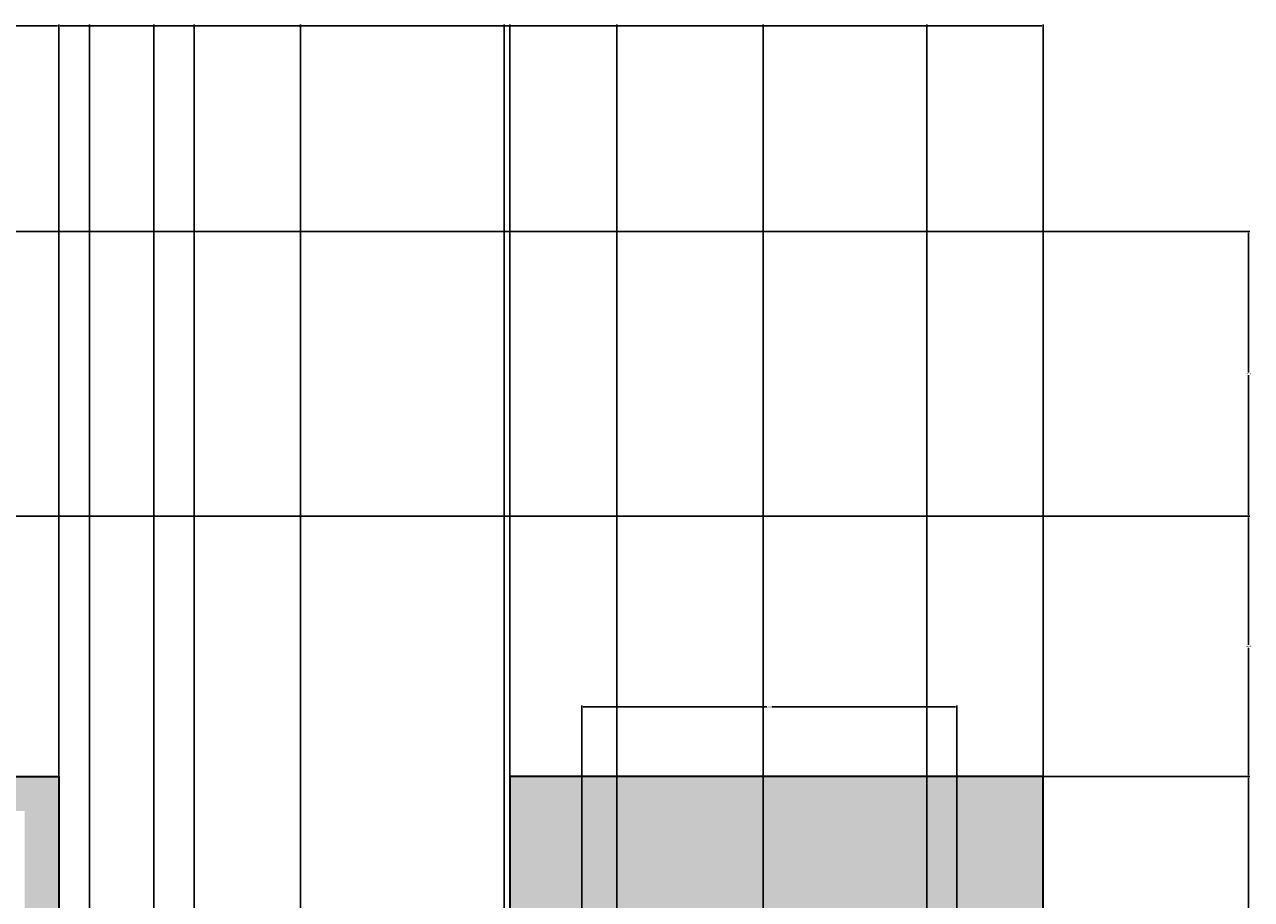
# Model space of a CAD drawing. Units: inches. Extents: x 73 to 607, y 92 to 651.
# Tile 18 of 18: x 446 to 607, y 536 to 651. Entities that reach past the tile are written whole.
import ezdxf

# ---------------------------------------------------------------- set-up
doc = ezdxf.new("R2010")
doc.units = ezdxf.units.IN
doc.header["$MEASUREMENT"] = 0
for name, color, linetype, lineweight in [('A-ANNO-DIMS', 2, 'Continuous', 18), ('A-ELEV', 7, 'Continuous', 35), ('A-ELEV-PATT-BKGD', 252, 'Continuous', 13), ('A-ELEV-PATT-WOOD', 32, 'Continuous', 13)]:
    doc.layers.add(name, color=color, linetype=linetype, lineweight=lineweight)
doc.styles.get("Standard").update_dxf_attribs({"font": 'arial.ttf'})
doc.dimstyles.get("Standard").update_dxf_attribs({"dimtxt": 0.18, "dimasz": 0.18, "dimexe": 0.18, "dimexo": 0.0625, "dimgap": 0.09, "dimtad": 0, "dimtih": 1, "dimtoh": 1, "dimdec": 4, "dimzin": 0, "dimdsep": 46, "dimtxsty": 'Standard', "dimcen": 0.09, "dimadec": 0, "dimazin": 0, "dimtfac": 1, "dimtdec": 4, "dimtofl": 0, "dimtmove": 0, "dimatfit": 3, "dimfxl": 1, "dimtolj": 1, "dimtzin": 0, "dimarcsym": 0})

# ---------------------------------------------------------------- blocks, each defined once
blk = doc.blocks.new('*D12')
at = {"layer": 'A-ANNO-DIMS', "color": 0, "lineweight": -2, "transparency": 16777216}
for p, q in [((394.78, 623.86), (394.78, 650.98)), ((394.96, 650.8), (422.33, 650.8)), ((450.48, 650.8), (423.11, 650.8)), ((450.66, 552.22), (450.66, 650.98))]:
    blk.add_line(p, q, dxfattribs=at)
at = {"layer": 'A-ANNO-DIMS', "color": 0, "transparency": 16777216}
for points in [[(394.96, 650.83), (394.96, 650.77), (394.78, 650.8)], [(450.48, 650.83), (450.48, 650.77), (450.66, 650.8)]]:
    blk.add_solid(points, dxfattribs=at)
at = {"layer": 'Defpoints', "color": 0, "transparency": 16777216}
for p in [(450.66, 650.8), (394.78, 623.8), (450.66, 552.16)]:
    blk.add_point(p, dxfattribs=at)
at = {"layer": 'A-ANNO-DIMS', "color": 0, "transparency": 16777216, "insert": (422.72, 650.8), "char_height": 0.18, "attachment_point": 5}
blk.add_mtext('\\A1;55.88', dxfattribs=at)
blk = doc.blocks.new('*D13')
at = {"layer": 'A-ANNO-DIMS', "color": 0, "lineweight": -2, "transparency": 16777216}
for p, q in [((450.66, 552.22), (450.66, 650.98)), ((450.84, 650.8), (479.94, 650.8)), ((509.79, 650.8), (480.69, 650.8)), ((509.97, 552.22), (509.97, 650.98))]:
    blk.add_line(p, q, dxfattribs=at)
at = {"layer": 'A-ANNO-DIMS', "color": 0, "transparency": 16777216}
for points in [[(450.84, 650.83), (450.84, 650.77), (450.66, 650.8)], [(509.79, 650.83), (509.79, 650.77), (509.97, 650.8)]]:
    blk.add_solid(points, dxfattribs=at)
at = {"layer": 'Defpoints', "color": 0, "transparency": 16777216}
for p in [(509.97, 650.8), (450.66, 552.16), (509.97, 552.16)]:
    blk.add_point(p, dxfattribs=at)
at = {"layer": 'A-ANNO-DIMS', "color": 0, "transparency": 16777216, "insert": (480.31, 650.8), "char_height": 0.18, "attachment_point": 5}
blk.add_mtext('\\A1;59.31', dxfattribs=at)
blk = doc.blocks.new('*D14')
at = {"layer": 'A-ANNO-DIMS', "color": 0, "lineweight": -2, "transparency": 16777216}
for p, q in [((509.97, 552.22), (509.97, 650.98)), ((510.15, 650.8), (544.64, 650.8)), ((579.92, 650.8), (545.43, 650.8)), ((580.1, 552.22), (580.1, 650.98))]:
    blk.add_line(p, q, dxfattribs=at)
at = {"layer": 'A-ANNO-DIMS', "color": 0, "transparency": 16777216}
for points in [[(510.15, 650.83), (510.15, 650.77), (509.97, 650.8)], [(579.92, 650.83), (579.92, 650.77), (580.1, 650.8)]]:
    blk.add_solid(points, dxfattribs=at)
at = {"layer": 'Defpoints', "color": 0, "transparency": 16777216}
for p in [(580.1, 650.8), (509.97, 552.16), (580.1, 552.16)]:
    blk.add_point(p, dxfattribs=at)
at = {"layer": 'A-ANNO-DIMS', "color": 0, "transparency": 16777216, "insert": (545.03, 650.8), "char_height": 0.18, "attachment_point": 5}
blk.add_mtext('\\A1;70.13', dxfattribs=at)
blk = doc.blocks.new('*D22')
at = {"layer": 'A-ANNO-DIMS', "color": 0, "lineweight": -2, "transparency": 16777216}
for p, q in [((580.16, 552.16), (607.28, 552.16)), ((607.1, 551.98), (607.1, 528.36)), ((607.1, 504.38), (607.1, 528)), ((510.03, 504.2), (607.28, 504.2))]:
    blk.add_line(p, q, dxfattribs=at)
at = {"layer": 'A-ANNO-DIMS', "color": 0, "transparency": 16777216}
for points in [[(607.07, 551.98), (607.13, 551.98), (607.1, 552.16)], [(607.07, 504.38), (607.13, 504.38), (607.1, 504.2)]]:
    blk.add_solid(points, dxfattribs=at)
at = {"layer": 'Defpoints', "color": 0, "transparency": 16777216}
for p in [(580.1, 552.16), (607.1, 552.16), (509.97, 504.2)]:
    blk.add_point(p, dxfattribs=at)
at = {"layer": 'A-ANNO-DIMS', "color": 0, "transparency": 16777216, "insert": (607.1, 528.18), "char_height": 0.18, "attachment_point": 5}
blk.add_mtext('\\A1;47.95', dxfattribs=at)
blk = doc.blocks.new('*D23')
at = {"layer": 'A-ANNO-DIMS', "color": 0, "lineweight": -2, "transparency": 16777216}
for p, q in [((394.84, 586.39), (607.28, 586.39)), ((607.1, 586.21), (607.1, 569.46)), ((607.1, 552.34), (607.1, 569.09)), ((580.16, 552.16), (607.28, 552.16))]:
    blk.add_line(p, q, dxfattribs=at)
at = {"layer": 'A-ANNO-DIMS', "color": 0, "transparency": 16777216}
for points in [[(607.07, 586.21), (607.13, 586.21), (607.1, 586.39)], [(607.07, 552.34), (607.13, 552.34), (607.1, 552.16)]]:
    blk.add_solid(points, dxfattribs=at)
at = {"layer": 'Defpoints', "color": 0, "transparency": 16777216}
for p in [(394.78, 586.39), (607.1, 586.39), (580.1, 552.16)]:
    blk.add_point(p, dxfattribs=at)
at = {"layer": 'A-ANNO-DIMS', "color": 0, "transparency": 16777216, "insert": (607.1, 569.28), "char_height": 0.18, "attachment_point": 5}
blk.add_mtext('\\A1;34.236', dxfattribs=at)
blk = doc.blocks.new('*D24')
at = {"layer": 'A-ANNO-DIMS', "color": 0, "lineweight": -2, "transparency": 16777216}
for p, q in [((394.84, 623.8), (607.28, 623.8)), ((607.1, 623.62), (607.1, 605.28)), ((607.1, 586.57), (607.1, 604.92)), ((394.84, 586.39), (607.28, 586.39))]:
    blk.add_line(p, q, dxfattribs=at)
at = {"layer": 'A-ANNO-DIMS', "color": 0, "transparency": 16777216}
for points in [[(607.07, 623.62), (607.13, 623.62), (607.1, 623.8)], [(607.07, 586.57), (607.13, 586.57), (607.1, 586.39)]]:
    blk.add_solid(points, dxfattribs=at)
at = {"layer": 'Defpoints', "color": 0, "transparency": 16777216}
for p in [(394.78, 623.8), (607.1, 623.8), (394.78, 586.39)]:
    blk.add_point(p, dxfattribs=at)
at = {"layer": 'A-ANNO-DIMS', "color": 0, "transparency": 16777216, "insert": (607.1, 605.1), "char_height": 0.18, "attachment_point": 5}
blk.add_mtext('\\A1;37.41', dxfattribs=at)
blk = doc.blocks.new('*D46')
at = {"layer": 'A-ANNO-DIMS', "color": 0, "lineweight": -2, "transparency": 16777216}
for p, q in [((450.6, 552.16), (423.48, 552.16)), ((423.66, 551.98), (423.66, 508.79)), ((423.66, 465.24), (423.66, 508.43)), ((450.6, 465.06), (423.48, 465.06))]:
    blk.add_line(p, q, dxfattribs=at)
at = {"layer": 'A-ANNO-DIMS', "color": 0, "transparency": 16777216}
for points in [[(423.63, 551.98), (423.69, 551.98), (423.66, 552.16)], [(423.63, 465.24), (423.69, 465.24), (423.66, 465.06)]]:
    blk.add_solid(points, dxfattribs=at)
at = {"layer": 'Defpoints', "color": 0, "transparency": 16777216}
for p in [(423.66, 552.16), (450.66, 552.16), (450.66, 465.06)]:
    blk.add_point(p, dxfattribs=at)
at = {"layer": 'A-ANNO-DIMS', "color": 0, "transparency": 16777216, "insert": (423.66, 508.61), "char_height": 0.18, "attachment_point": 5}
blk.add_mtext('\\A1;87.1', dxfattribs=at)
blk = doc.blocks.new('*D48')
at = {"layer": 'A-ANNO-DIMS', "color": 0, "lineweight": -2, "transparency": 16777216}
for p, q in [((519.42, 534.37), (519.42, 561.49)), ((568.72, 534.37), (568.72, 561.49)), ((519.6, 561.31), (543.75, 561.31)), ((568.54, 561.31), (544.4, 561.31))]:
    blk.add_line(p, q, dxfattribs=at)
at = {"layer": 'A-ANNO-DIMS', "color": 0, "transparency": 16777216}
for points in [[(519.6, 561.34), (519.6, 561.28), (519.42, 561.31)], [(568.54, 561.34), (568.54, 561.28), (568.72, 561.31)]]:
    blk.add_solid(points, dxfattribs=at)
at = {"layer": 'Defpoints', "color": 0, "transparency": 16777216}
for p in [(568.72, 561.31), (519.42, 534.31), (568.72, 534.31)]:
    blk.add_point(p, dxfattribs=at)
at = {"layer": 'A-ANNO-DIMS', "color": 0, "transparency": 16777216, "insert": (544.07, 561.31), "char_height": 0.18, "attachment_point": 5}
blk.add_mtext('\\A1;49.3', dxfattribs=at)
blk = doc.blocks.new('*D103')
at = {"layer": 'A-ANNO-DIMS', "color": 0, "lineweight": -2, "transparency": 16777216}
for p, q in [((454.7, 256.69), (454.7, 650.98)), ((454.88, 650.8), (458.55, 650.8)), ((463, 650.8), (459.34, 650.8)), ((463.18, 243.92), (463.18, 650.98))]:
    blk.add_line(p, q, dxfattribs=at)
at = {"layer": 'A-ANNO-DIMS', "color": 0, "transparency": 16777216}
for points in [[(454.88, 650.83), (454.88, 650.77), (454.7, 650.8)], [(463, 650.83), (463, 650.77), (463.18, 650.8)]]:
    blk.add_solid(points, dxfattribs=at)
at = {"layer": 'Defpoints', "color": 0, "transparency": 16777216}
for p in [(463.18, 650.8), (454.7, 256.63), (463.18, 243.86)]:
    blk.add_point(p, dxfattribs=at)
at = {"layer": 'A-ANNO-DIMS', "color": 0, "transparency": 16777216, "insert": (458.94, 650.8), "char_height": 0.18, "attachment_point": 5}
blk.add_mtext('\\A1;8.475', dxfattribs=at)
blk = doc.blocks.new('*D104')
at = {"layer": 'A-ANNO-DIMS', "color": 0, "lineweight": -2, "transparency": 16777216}
for p, q in [((463.18, 243.92), (463.18, 650.98)), ((463.36, 650.8), (465.44, 650.8)), ((468.3, 650.8), (466.23, 650.8)), ((468.48, 225.79), (468.48, 650.98))]:
    blk.add_line(p, q, dxfattribs=at)
at = {"layer": 'A-ANNO-DIMS', "color": 0, "transparency": 16777216}
for points in [[(463.36, 650.83), (463.36, 650.77), (463.18, 650.8)], [(468.3, 650.83), (468.3, 650.77), (468.48, 650.8)]]:
    blk.add_solid(points, dxfattribs=at)
at = {"layer": 'Defpoints', "color": 0, "transparency": 16777216}
for p in [(468.48, 650.8), (463.18, 243.86), (468.48, 225.73)]:
    blk.add_point(p, dxfattribs=at)
at = {"layer": 'A-ANNO-DIMS', "color": 0, "transparency": 16777216, "insert": (465.83, 650.8), "char_height": 0.18, "attachment_point": 5}
blk.add_mtext('\\A1;5.304', dxfattribs=at)
blk = doc.blocks.new('*D105')
at = {"layer": 'A-ANNO-DIMS', "color": 0, "lineweight": -2, "transparency": 16777216}
for p, q in [((468.48, 225.79), (468.48, 650.98)), ((468.66, 650.8), (475.01, 650.8)), ((482.26, 650.8), (475.92, 650.8)), ((482.44, 246.99), (482.44, 650.98))]:
    blk.add_line(p, q, dxfattribs=at)
at = {"layer": 'A-ANNO-DIMS', "color": 0, "transparency": 16777216}
for points in [[(468.66, 650.83), (468.66, 650.77), (468.48, 650.8)], [(482.26, 650.83), (482.26, 650.77), (482.44, 650.8)]]:
    blk.add_solid(points, dxfattribs=at)
at = {"layer": 'Defpoints', "color": 0, "transparency": 16777216}
for p in [(482.44, 650.8), (482.44, 246.92), (468.48, 225.73)]:
    blk.add_point(p, dxfattribs=at)
at = {"layer": 'A-ANNO-DIMS', "color": 0, "transparency": 16777216, "insert": (475.46, 650.8), "char_height": 0.18, "attachment_point": 5}
blk.add_mtext('\\A1;13.957', dxfattribs=at)
blk = doc.blocks.new('*D106')
at = {"layer": 'A-ANNO-DIMS', "color": 0, "lineweight": -2, "transparency": 16777216}
for p, q in [((482.44, 246.99), (482.44, 650.98)), ((482.62, 650.8), (495.37, 650.8)), ((509.06, 650.8), (496.3, 650.8)), ((509.24, 232.76), (509.24, 650.98))]:
    blk.add_line(p, q, dxfattribs=at)
at = {"layer": 'A-ANNO-DIMS', "color": 0, "transparency": 16777216}
for points in [[(482.62, 650.83), (482.62, 650.77), (482.44, 650.8)], [(509.06, 650.83), (509.06, 650.77), (509.24, 650.8)]]:
    blk.add_solid(points, dxfattribs=at)
at = {"layer": 'Defpoints', "color": 0, "transparency": 16777216}
for p in [(509.24, 650.8), (482.44, 246.92), (509.24, 232.7)]:
    blk.add_point(p, dxfattribs=at)
at = {"layer": 'A-ANNO-DIMS', "color": 0, "transparency": 16777216, "insert": (495.84, 650.8), "char_height": 0.18, "attachment_point": 5}
blk.add_mtext('\\A1;26.797', dxfattribs=at)
blk = doc.blocks.new('*D107')
at = {"layer": 'A-ANNO-DIMS', "color": 0, "lineweight": -2, "transparency": 16777216}
for p, q in [((509.24, 232.76), (509.24, 650.98)), ((509.42, 650.8), (516.18, 650.8)), ((523.85, 650.8), (517.09, 650.8)), ((524.03, 250.33), (524.03, 650.98))]:
    blk.add_line(p, q, dxfattribs=at)
at = {"layer": 'A-ANNO-DIMS', "color": 0, "transparency": 16777216}
for points in [[(509.42, 650.83), (509.42, 650.77), (509.24, 650.8)], [(523.85, 650.83), (523.85, 650.77), (524.03, 650.8)]]:
    blk.add_solid(points, dxfattribs=at)
at = {"layer": 'Defpoints', "color": 0, "transparency": 16777216}
for p in [(524.03, 650.8), (524.03, 250.27), (509.24, 232.7)]:
    blk.add_point(p, dxfattribs=at)
at = {"layer": 'A-ANNO-DIMS', "color": 0, "transparency": 16777216, "insert": (516.63, 650.8), "char_height": 0.18, "attachment_point": 5}
blk.add_mtext('\\A1;14.794', dxfattribs=at)
blk = doc.blocks.new('*D108')
at = {"layer": 'A-ANNO-DIMS', "color": 0, "lineweight": -2, "transparency": 16777216}
for p, q in [((524.03, 250.33), (524.03, 650.98)), ((524.21, 650.8), (533.28, 650.8)), ((543.11, 650.8), (534.05, 650.8)), ((543.29, 226.9), (543.29, 650.98))]:
    blk.add_line(p, q, dxfattribs=at)
at = {"layer": 'A-ANNO-DIMS', "color": 0, "transparency": 16777216}
for points in [[(524.21, 650.83), (524.21, 650.77), (524.03, 650.8)], [(543.11, 650.83), (543.11, 650.77), (543.29, 650.8)]]:
    blk.add_solid(points, dxfattribs=at)
at = {"layer": 'Defpoints', "color": 0, "transparency": 16777216}
for p in [(543.29, 650.8), (524.03, 250.27), (543.29, 226.84)]:
    blk.add_point(p, dxfattribs=at)
at = {"layer": 'A-ANNO-DIMS', "color": 0, "transparency": 16777216, "insert": (533.66, 650.8), "char_height": 0.18, "attachment_point": 5}
blk.add_mtext('\\A1;19.26', dxfattribs=at)
blk = doc.blocks.new('*D109')
at = {"layer": 'A-ANNO-DIMS', "color": 0, "lineweight": -2, "transparency": 16777216}
for p, q in [((543.29, 226.9), (543.29, 650.98)), ((543.47, 650.8), (553.57, 650.8)), ((564.61, 650.8), (554.5, 650.8)), ((564.79, 245.31), (564.79, 650.98))]:
    blk.add_line(p, q, dxfattribs=at)
at = {"layer": 'A-ANNO-DIMS', "color": 0, "transparency": 16777216}
for points in [[(543.47, 650.83), (543.47, 650.77), (543.29, 650.8)], [(564.61, 650.83), (564.61, 650.77), (564.79, 650.8)]]:
    blk.add_solid(points, dxfattribs=at)
at = {"layer": 'Defpoints', "color": 0, "transparency": 16777216}
for p in [(564.79, 650.8), (564.79, 245.25), (543.29, 226.84)]:
    blk.add_point(p, dxfattribs=at)
at = {"layer": 'A-ANNO-DIMS', "color": 0, "transparency": 16777216, "insert": (554.04, 650.8), "char_height": 0.18, "attachment_point": 5}
blk.add_mtext('\\A1;21.493', dxfattribs=at)

msp = doc.modelspace()

# ---------------------------------------------------------------- hatches: boundary and pattern name
at = {"layer": 'A-ELEV-PATT-BKGD'}
h = msp.add_hatch(color=256, dxfattribs=at)
h.dxf.hatch_style = 1
h.paths.add_polyline_path([(321.3008, 479.2042), (312.3008, 479.2042), (312.3008, 478.7576), (312.3008, 412.636), (321.3008, 412.636)])
h.paths.add_polyline_path([(312.3008, 504.7576), (256.4726, 504.7576), (256.4726, 503.4576), (312.3008, 503.4576)], flags=17)
h.paths.add_polyline_path([(321.3008, 543.1576), (321.3008, 552.1576), (320.3257, 552.1576), (312.3008, 552.1576), (256.4726, 552.1576), (256.4726, 543.1576), (312.3008, 543.1576), (312.3008, 479.2042), (321.3008, 479.2042)])
h.paths.add_polyline_path([(451.5214, 412.636), (256.4726, 412.636), (256.4726, 403.636), (442.5214, 403.636), (442.5214, 320.2042), (206.1343, 320.2042), (206.1343, 320.9135), (206.1343, 403.636), (256.4726, 403.636), (256.4726, 412.636), (201.6343, 412.636), (201.6343, 320.9135), (201.6343, 320.2042), (201.6343, 311.2042), (256.4726, 311.2042), (451.5214, 311.2042)])
h.paths.add_polyline_path([(431.07, 258.6914), (369.5339, 258.6914), (369.5339, 247.4054), (396.692, 247.4054), (425.07, 247.4054), (425.07, 194.7312), (396.692, 194.6197), (396.692, 194.5366), (369.5339, 194.5366), (369.5339, 185.6619), (431.07, 185.6619)])
h.paths.add_polyline_path([(580.0983, 262.3024), (451.5214, 262.3024), (451.5214, 143.2042), (580.0983, 143.2042)])
h.paths.add_polyline_path([(454.7049, 174.802), (454.7049, 256.6321), (577.9249, 256.6321), (577.9249, 174.802)], flags=16)
h.paths.add_polyline_path([(465.9716, 191.1416, -1), (473.7874, 191.1416, -1)], flags=0)
h.paths.add_polyline_path([(490.5373, 181.6586, -1), (494.9999, 181.6586, -1)], flags=0)
h.paths.add_polyline_path([(476.2996, 209.8287, -1), (500.5844, 209.8287, -1)], flags=0)
h.paths.add_polyline_path([(505.3326, 194.7675, -1), (512.5843, 194.7675, -1)], flags=0)
h.paths.add_polyline_path([(520.9613, 186.679, -1), (526.544, 186.679, -1)], flags=0)
h.paths.add_polyline_path([(466.8103, 225.7267, -1), (470.1573, 225.7267, -1)], flags=0)
h.paths.add_polyline_path([(527.1059, 203.6926, -1), (536.0311, 203.6926, -1)], flags=0)
h.paths.add_polyline_path([(504.775, 232.6995, -1), (513.7002, 232.6995, -1)], flags=0)
h.paths.add_polyline_path([(546.9241, 183.611, -1), (554.7336, 183.611, -1)], flags=0)
h.paths.add_polyline_path([(459.5544, 243.856, -1), (466.8061, 243.856, -1)], flags=0)
h.paths.add_polyline_path([(476.3045, 246.924, -1), (488.5767, 246.924, -1)], flags=0)
h.paths.add_polyline_path([(529.9044, 226.8424, -1), (556.68, 226.8424, -1)], flags=0)
h.paths.add_polyline_path([(554.1814, 203.9716, -1), (561.4331, 203.9716, -1)], flags=0)
h.paths.add_polyline_path([(567.8561, 193.3729, -1), (570.6475, 193.3729, -1)], flags=0)
h.paths.add_polyline_path([(522.3584, 250.271, -1), (525.7053, 250.271, -1)], flags=0)
h.paths.add_polyline_path([(561.9965, 245.2506, -1), (567.5748, 245.2506, -1)], flags=0)
h.paths.add_polyline_path([(347.8686, 194.5366), (341.8686, 194.5366), (341.8686, 194.5452), (314.0144, 194.5452), (314.0144, 188.5452), (347.8686, 188.5452)])
h.paths.add_polyline_path([(347.8686, 253.4054), (314.0144, 253.4054), (314.0144, 247.4054), (341.8686, 247.4054), (347.8686, 247.4054)])
h.paths.add_polyline_path([(304.3559, 253.4054), (298.3559, 253.4054), (298.3559, 188.5452), (304.3559, 188.5452)])
h.paths.add_polyline_path([(450.6603, 552.1576), (369.9727, 552.1576), (369.9727, 479.2042), (374.4727, 479.2042), (374.4727, 547.6576), (446.1603, 547.6576), (446.1603, 479.2042), (450.6603, 479.2042)])
h.paths.add_polyline_path([(374.4727, 479.2042), (369.9727, 479.2042), (369.9727, 465.0632), (374.4727, 465.0632)])
h.paths.add_polyline_path([(450.6603, 479.2042), (446.1603, 479.2042), (446.1603, 465.0632), (450.6603, 465.0632)])
h.paths.add_polyline_path([(256.4726, 281.6039), (109.0983, 281.6039), (100.0983, 281.6039), (100.0983, 167.2042), (100.0983, 143.2042), (109.0983, 143.2042), (109.0983, 167.2042), (109.0983, 272.6039), (256.4726, 272.6039)])
at = {"layer": 'A-ELEV-PATT-WOOD'}
h = msp.add_hatch(color=256, dxfattribs=at)
h.dxf.hatch_style = 1
h.paths.add_polyline_path([(580.0983, 552.1576), (509.9692, 552.1576), (509.9692, 311.2042), (580.0983, 311.2042)])
h.paths.add_polyline_path([(568.7235, 534.3065), (568.7235, 325.2318), (519.4225, 325.2318), (519.4225, 534.3065)], flags=16)
h.paths.add_polyline_path([(526.0397, 406.6944), (561.5694, 406.6944), (561.5694, 370.0444), (526.0397, 370.0444)], flags=0)
h.paths.add_polyline_path([(528.0397, 404.6944), (559.5694, 404.6944), (559.5694, 372.0444), (528.0397, 372.0444)], flags=0)
h.paths.add_polyline_path([(568.7235, 534.3065), (519.4225, 534.3065), (519.4225, 530.3065), (568.7235, 530.3065)], flags=0)
h.paths.add_polyline_path([(568.7235, 530.3065), (519.4225, 530.3065), (519.4225, 526.3065), (568.7235, 526.3065)], flags=0)

# ---------------------------------------------------------------- linework, layer by layer
at = {"layer": 'A-ELEV'}
for p, q in [((369.9727, 552.1576), (450.6603, 552.1576)), ((450.6603, 552.1576), (450.6603, 465.0632))]:
    msp.add_line(p, q, dxfattribs=at)
msp.add_lwpolyline([(509.9692, 311.2042), (580.0983, 311.2042), (580.0983, 552.1576), (509.9692, 552.1576)], close=True, dxfattribs=at)

# ---------------------------------------------------------------- dimensions: what is measured, and where the dimension line sits
at = {"layer": 'A-ANNO-DIMS'}
for base, p1, p2, override, picture, middle in [((450.6603, 650.801), (394.7799, 623.801), (450.6603, 552.1576), {"dimdec": 2, "dimlfac": 1, "dimrnd": 0, "dimzin": 0, "dimdsep": 46, "dimlunit": 2}, '*D12', (422.7201, 650.801)), ((509.9692, 650.801), (450.6603, 552.1576), (509.9692, 552.1576), {"dimdec": 2, "dimlfac": 1, "dimrnd": 0, "dimzin": 0, "dimdsep": 46, "dimlunit": 2}, '*D13', (480.3148, 650.801)), ((463.1802, 650.801), (454.7049, 256.6321), (463.1802, 243.856), {"dimdec": 3, "dimlfac": 1, "dimrnd": 0, "dimzin": 0, "dimdsep": 46, "dimlunit": 2}, '*D103', (458.9425, 650.801)), ((468.4838, 650.801), (463.1802, 243.856), (468.4838, 225.7267), {"dimdec": 3, "dimlfac": 1, "dimrnd": 0, "dimzin": 0, "dimdsep": 46, "dimlunit": 2}, '*D104', (465.832, 650.801)), ((482.4406, 650.801), (468.4838, 225.7267), (482.4406, 246.924), {"dimdec": 3, "dimlfac": 1, "dimrnd": 0, "dimzin": 0, "dimdsep": 46, "dimlunit": 2}, '*D105', (475.4622, 650.801)), ((509.2376, 650.801), (482.4406, 246.924), (509.2376, 232.6995), {"dimdec": 3, "dimlfac": 1, "dimrnd": 0, "dimzin": 0, "dimdsep": 46, "dimlunit": 2}, '*D106', (495.8391, 650.801)), ((524.0318, 650.801), (509.2376, 232.6995), (524.0318, 250.271), {"dimdec": 3, "dimlfac": 1, "dimrnd": 0, "dimzin": 0, "dimdsep": 46, "dimlunit": 2}, '*D107', (516.6347, 650.801)), ((580.0983, 650.801), (509.9692, 552.1576), (580.0983, 552.1576), {"dimdec": 2, "dimlfac": 1, "dimrnd": 0, "dimzin": 0, "dimdsep": 46, "dimlunit": 2}, '*D14', (545.0338, 650.801)), ((543.2922, 650.801), (524.0318, 250.271), (543.2922, 226.8424), {"dimdec": 2, "dimlfac": 1, "dimrnd": 0, "dimzin": 0, "dimdsep": 46, "dimlunit": 2}, '*D108', (533.662, 650.801)), ((564.7856, 650.801), (543.2922, 226.8424), (564.7856, 245.2506), {"dimdec": 3, "dimlfac": 1, "dimrnd": 0, "dimzin": 0, "dimdsep": 46, "dimlunit": 2}, '*D109', (554.0389, 650.801)), ((568.7235, 561.3065), (519.4225, 534.3065), (568.7235, 534.3065), {"dimdec": 1, "dimlfac": 1, "dimrnd": 0, "dimzin": 0, "dimdsep": 46, "dimlunit": 2}, '*D48', (544.073, 561.3065))]:
    dim = msp.add_linear_dim(base=base, p1=p1, p2=p2, dimstyle='Standard', override=override, dxfattribs=at)
    dim.commit()
    dim.dimension.update_dxf_attribs({"geometry": picture, "text_midpoint": middle})
for base, p1, p2, override, picture, middle in [((607.0983, 623.801), (394.7799, 586.3933), (394.7799, 623.801), {"dimdec": 2, "dimlfac": 1, "dimrnd": 0, "dimzin": 0, "dimdsep": 46, "dimlunit": 2}, '*D24', (607.0983, 605.0972)), ((607.0983, 586.3933), (580.0983, 552.1576), (394.7799, 586.3933), {"dimdec": 3, "dimlfac": 1, "dimrnd": 0, "dimzin": 0, "dimdsep": 46, "dimlunit": 2}, '*D23', (607.0983, 569.2755)), ((423.6603, 552.1576), (450.6603, 465.0632), (450.6603, 552.1576), {"dimdec": 1, "dimlfac": 1, "dimrnd": 0, "dimzin": 0, "dimdsep": 46, "dimlunit": 2}, '*D46', (423.6603, 508.6104)), ((607.0983, 552.1576), (509.9692, 504.2042), (580.0983, 552.1576), {"dimdec": 2, "dimlfac": 1, "dimrnd": 0, "dimzin": 0, "dimdsep": 46, "dimlunit": 2}, '*D22', (607.0983, 528.1809))]:
    dim = msp.add_linear_dim(base=base, p1=p1, p2=p2, angle=90, dimstyle='Standard', override=override, dxfattribs=at)
    dim.commit()
    dim.dimension.update_dxf_attribs({"geometry": picture, "text_midpoint": middle})

doc.saveas('drawing.dxf')
